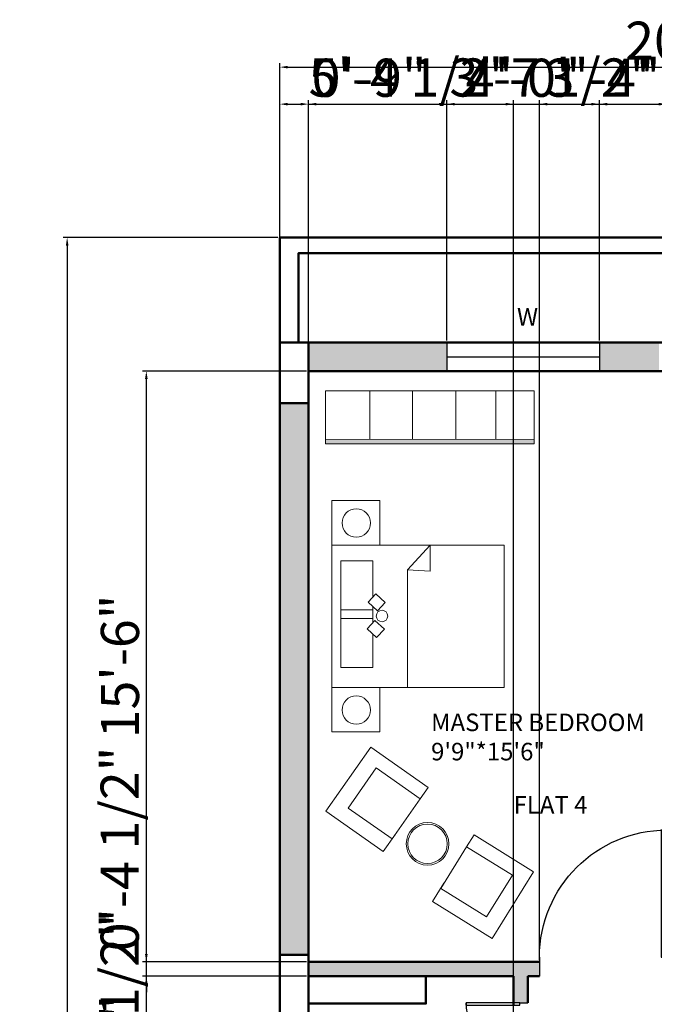
# Model space of a CAD drawing. Units: inches. Extents: x 2063 to 3370, y 2091 to 2971.
# Tile 13 of 14: x 2986 to 3185, y 2623 to 2933. Entities that reach past the tile are written whole.
import ezdxf

# ---------------------------------------------------------------- set-up
doc = ezdxf.new("R2010")
doc.units = ezdxf.units.IN
for name, color, linetype, lineweight in [('A-ANNO-DIMS', 2, 'Continuous', 18), ('A-ANNO-TEXT', 7, 'Continuous', 18), ('A-AREA-IDEN', 3, 'Continuous', 18), ('A-COLS', 7, 'Continuous', 50), ('A-DOOR', 4, 'Continuous', 25), ('A-FURN', 8, 'Continuous', 18), ('A-GLAZ', 131, 'Continuous', 25), ('A-WALL', 7, 'Continuous', 50), ('A-WALL-PATT', 8, 'Continuous', 13)]:
    doc.layers.add(name, color=color, linetype=linetype, lineweight=lineweight)
doc.styles.get("Standard").update_dxf_attribs({"font": 'arial.ttf'})
doc.dimstyles.new('ISO-25', dxfattribs={"dimtxt": 12, "dimasz": 2.5, "dimexe": 1.25, "dimexo": 0.625, "dimtad": 1, "dimdec": 0, "dimlunit": 4, "dimtxsty": 'Standard', "dimcen": 2.5, "dimadec": 0, "dimazin": 0, "dimtfac": 1, "dimtdec": 0, "dimtmove": 0, "dimatfit": 3, "dimfxl": 1, "dimarcsym": 0})

# ---------------------------------------------------------------- blocks, each defined once
blk = doc.blocks.new('*D9')
at = {"layer": 'A-ANNO-DIMS', "color": 0, "lineweight": -2, "transparency": 16777216}
for p, q in [((3067.42, 2865.05), (3067.42, 2919.33)), ((3069.92, 2918.08), (3304.92, 2918.08)), ((3307.42, 2865.05), (3307.42, 2919.33))]:
    blk.add_line(p, q, dxfattribs=at)
at = {"layer": 'A-ANNO-DIMS', "color": 0, "transparency": 16777216}
for points in [[(3069.92, 2918.5), (3069.92, 2917.67), (3067.42, 2918.08)], [(3304.92, 2918.5), (3304.92, 2917.67), (3307.42, 2918.08)]]:
    blk.add_solid(points, dxfattribs=at)
at = {"layer": 'Defpoints', "color": 0, "transparency": 16777216}
for p in [(3307.42, 2918.08), (3067.42, 2864.43), (3307.42, 2864.43)]:
    blk.add_point(p, dxfattribs=at)
at = {"layer": 'A-ANNO-DIMS', "color": 0, "transparency": 16777216, "insert": (3187.42, 2924.84), "char_height": 12, "attachment_point": 5}
blk.add_mtext("20'", dxfattribs=at)
blk = doc.blocks.new('*D10')
at = {"layer": 'A-ANNO-DIMS', "color": 0, "lineweight": -2, "transparency": 16777216}
for p, q in [((3066.79, 2864.43), (2999.25, 2864.43)), ((3000.5, 2861.93), (3000.5, 2146.93)), ((3066.79, 2144.43), (2999.25, 2144.43))]:
    blk.add_line(p, q, dxfattribs=at)
at = {"layer": 'A-ANNO-DIMS', "color": 0, "transparency": 16777216}
for points in [[(3000.09, 2861.93), (3000.92, 2861.93), (3000.5, 2864.43)], [(3000.09, 2146.93), (3000.92, 2146.93), (3000.5, 2144.43)]]:
    blk.add_solid(points, dxfattribs=at)
at = {"layer": 'Defpoints', "color": 0, "transparency": 16777216}
for p in [(3067.42, 2864.43), (3000.5, 2144.43), (3067.42, 2144.43)]:
    blk.add_point(p, dxfattribs=at)
at = {"layer": 'A-ANNO-DIMS', "color": 0, "transparency": 16777216, "insert": (2993.75, 2504.43), "char_height": 12, "attachment_point": 5, "rotation": 90}
blk.add_mtext("60'", dxfattribs=at)
blk = doc.blocks.new('*U2')
for p, q in [((0, 0), (0, -6)), ((40, 0), (40, -6))]:
    blk.add_line(p, q)
blk.add_lwpolyline([(0, 0), (0, 40), (1.75, 40), (1.75, 0)], close=True)
blk.add_arc((0, 0), 40, 0, 90)
blk = doc.blocks.new('BED-DOUBLE')
for p, q in [((23.79, 50.98), (30.96, 58.78)), ((30.96, 58.78), (30.96, 50.54)), ((23.79, 14), (23.79, 50.98)), ((30.96, 50.54), (23.79, 50.98))]:
    blk.add_line(p, q)
for points in [[(0, 58.78), (15.11, 58.78), (15.11, 72.78), (0, 72.78)], [(0, 58.78), (54.26, 58.78), (54.26, 14), (0, 14)], [(11.45, 40.86), (13.89, 43.46), (16.84, 40.71), (14.4, 38.1)], [(11.16, 32.43), (13.59, 35.03), (16.54, 32.28), (14.11, 29.67)], [(0, 0), (15.11, 0), (15.11, 14), (0, 14)]]:
    blk.add_lwpolyline(points, close=True)
for points in [[(12.88, 42.39), (12.88, 53.87), (2.9, 53.87), (2.9, 35.71), (12.88, 35.71), (12.88, 39.52)], [(12.88, 34.27), (12.88, 38.39), (2.9, 38.39), (2.9, 20.23), (12.88, 20.23), (12.88, 30.81)]]:
    blk.add_lwpolyline(points)
for centre, radius in [((7.71, 65.74), 4.47), ((15.81, 36.46), 1.81), ((7.71, 6.86), 4.47)]:
    blk.add_circle(centre, radius)
blk = doc.blocks.new('WARDROBE')
for p, q in [((13.88, 1.44), (13.88, 16.75)), ((27.33, 1.44), (27.33, 16.75)), ((40.97, 1.44), (40.97, 16.75)), ((53.56, 1.44), (53.56, 16.75)), ((0, 1.42), (65.55, 1.52))]:
    blk.add_line(p, q)
blk.add_lwpolyline([(0, 16.75), (65.55, 16.75), (65.55, 0), (0, 0)], close=True)
blk = doc.blocks.new('ARMCHAIR')
for p, q in [((10.7, 28.87), (13.03, 32.61)), ((13.03, 32.61), (31.78, 20.96)), ((31.78, 20.96), (18.75, 0)), ((0, 11.65), (3.54, 17.35)), ((18.75, 0), (0, 11.65))]:
    blk.add_line(p, q)
blk.add_lwpolyline([(2.55, 15.75), (16.92, 6.82), (25.07, 19.93), (10.7, 28.87)], close=True)
blk = doc.blocks.new('*D135')
at = {"layer": 'A-ANNO-DIMS', "color": 0, "lineweight": -2, "transparency": 16777216}
for p, q in [((3067.42, 2832.05), (3067.42, 2907.68)), ((3076.42, 2823.05), (3076.42, 2907.68)), ((3069.92, 2906.43), (3073.92, 2906.43)), ((3076.42, 2906.43), (3112.06, 2906.43))]:
    blk.add_line(p, q, dxfattribs=at)
at = {"layer": 'A-ANNO-DIMS', "color": 0, "transparency": 16777216}
for points in [[(3069.92, 2906.84), (3069.92, 2906.01), (3067.42, 2906.43)], [(3073.92, 2906.84), (3073.92, 2906.01), (3076.42, 2906.43)]]:
    blk.add_solid(points, dxfattribs=at)
at = {"layer": 'Defpoints', "color": 0, "transparency": 16777216}
for p in [(3076.42, 2906.43), (3067.42, 2831.43), (3076.42, 2822.43)]:
    blk.add_point(p, dxfattribs=at)
at = {"layer": 'A-ANNO-DIMS', "color": 0, "transparency": 16777216, "insert": (3095.49, 2913.18), "char_height": 12, "attachment_point": 5}
blk.add_mtext('0\'-9"', dxfattribs=at)
blk = doc.blocks.new('*D136')
at = {"layer": 'A-ANNO-DIMS', "color": 0, "lineweight": -2, "transparency": 16777216}
for p, q in [((3076.42, 2823.05), (3076.42, 2907.68)), ((3119.94, 2832.05), (3119.94, 2907.68)), ((3078.92, 2906.43), (3117.44, 2906.43)), ((3119.94, 2906.43), (3183.54, 2906.43))]:
    blk.add_line(p, q, dxfattribs=at)
at = {"layer": 'A-ANNO-DIMS', "color": 0, "transparency": 16777216}
for points in [[(3078.92, 2906.84), (3078.92, 2906.01), (3076.42, 2906.43)], [(3117.44, 2906.84), (3117.44, 2906.01), (3119.94, 2906.43)]]:
    blk.add_solid(points, dxfattribs=at)
at = {"layer": 'Defpoints', "color": 0, "transparency": 16777216}
for p in [(3119.94, 2906.43), (3119.94, 2831.43), (3076.42, 2822.43)]:
    blk.add_point(p, dxfattribs=at)
at = {"layer": 'A-ANNO-DIMS', "color": 0, "transparency": 16777216, "insert": (3152.99, 2913.26), "char_height": 12, "attachment_point": 5}
blk.add_mtext('3\'-7 1/2"', dxfattribs=at)
blk = doc.blocks.new('*D137')
at = {"layer": 'A-ANNO-DIMS', "color": 0, "lineweight": -2, "transparency": 16777216}
for p, q in [((3119.94, 2832.05), (3119.94, 2907.68)), ((3167.94, 2832.05), (3167.94, 2907.68)), ((3122.44, 2906.43), (3165.44, 2906.43))]:
    blk.add_line(p, q, dxfattribs=at)
at = {"layer": 'A-ANNO-DIMS', "color": 0, "transparency": 16777216}
for points in [[(3122.44, 2906.84), (3122.44, 2906.01), (3119.94, 2906.43)], [(3165.44, 2906.84), (3165.44, 2906.01), (3167.94, 2906.43)]]:
    blk.add_solid(points, dxfattribs=at)
at = {"layer": 'Defpoints', "color": 0, "transparency": 16777216}
for p in [(3167.94, 2906.43), (3119.94, 2831.43), (3167.94, 2831.43)]:
    blk.add_point(p, dxfattribs=at)
at = {"layer": 'A-ANNO-DIMS', "color": 0, "transparency": 16777216, "insert": (3143.94, 2913.18), "char_height": 12, "attachment_point": 5}
blk.add_mtext('4\'-0"', dxfattribs=at)
blk = doc.blocks.new('*D138')
at = {"layer": 'A-ANNO-DIMS', "color": 0, "lineweight": -2, "transparency": 16777216}
for p, q in [((3167.94, 2832.05), (3167.94, 2907.68)), ((3193.42, 2823.05), (3193.42, 2907.68)), ((3170.44, 2906.43), (3190.92, 2906.43)), ((3193.42, 2906.43), (3257.23, 2906.43))]:
    blk.add_line(p, q, dxfattribs=at)
at = {"layer": 'A-ANNO-DIMS', "color": 0, "transparency": 16777216}
for points in [[(3170.44, 2906.84), (3170.44, 2906.01), (3167.94, 2906.43)], [(3190.92, 2906.84), (3190.92, 2906.01), (3193.42, 2906.43)]]:
    blk.add_solid(points, dxfattribs=at)
at = {"layer": 'Defpoints', "color": 0, "transparency": 16777216}
for p in [(3193.42, 2906.43), (3167.94, 2831.43), (3193.42, 2822.43)]:
    blk.add_point(p, dxfattribs=at)
at = {"layer": 'A-ANNO-DIMS', "color": 0, "transparency": 16777216, "insert": (3226.57, 2913.26), "char_height": 12, "attachment_point": 5}
blk.add_mtext('2\'-1 1/2"', dxfattribs=at)
blk = doc.blocks.new('*D148')
at = {"layer": 'A-ANNO-DIMS', "color": 0, "lineweight": -2, "transparency": 16777216}
for p, q in [((3076.42, 2584.55), (3076.42, 2907.68)), ((3140.92, 2584.55), (3140.92, 2907.68)), ((3078.92, 2906.43), (3138.42, 2906.43))]:
    blk.add_line(p, q, dxfattribs=at)
at = {"layer": 'A-ANNO-DIMS', "color": 0, "transparency": 16777216}
for points in [[(3078.92, 2906.84), (3078.92, 2906.01), (3076.42, 2906.43)], [(3138.42, 2906.84), (3138.42, 2906.01), (3140.92, 2906.43)]]:
    blk.add_solid(points, dxfattribs=at)
at = {"layer": 'Defpoints', "color": 0, "transparency": 16777216}
for p in [(3140.92, 2906.43), (3076.42, 2583.93), (3140.92, 2583.93)]:
    blk.add_point(p, dxfattribs=at)
at = {"layer": 'A-ANNO-DIMS', "color": 0, "transparency": 16777216, "insert": (3108.67, 2913.26), "char_height": 12, "attachment_point": 5}
blk.add_mtext('5\'-4 1/2"', dxfattribs=at)
blk = doc.blocks.new('*D156')
at = {"layer": 'A-ANNO-DIMS', "color": 0, "lineweight": -2, "transparency": 16777216}
for p, q in [((3025.42, 2586.43), (3025.42, 2650.04)), ((3075.79, 2583.93), (3024.17, 2583.93)), ((3025.42, 2579.43), (3025.42, 2583.93)), ((3075.79, 2579.43), (3024.17, 2579.43)), ((3025.42, 2576.93), (3025.42, 2574.43))]:
    blk.add_line(p, q, dxfattribs=at)
at = {"layer": 'A-ANNO-DIMS', "color": 0, "transparency": 16777216}
for points in [[(3025, 2586.43), (3025.83, 2586.43), (3025.42, 2583.93)], [(3025, 2576.93), (3025.83, 2576.93), (3025.42, 2579.43)]]:
    blk.add_solid(points, dxfattribs=at)
at = {"layer": 'Defpoints', "color": 0, "transparency": 16777216}
for p in [(3025.42, 2583.93), (3076.42, 2583.93), (3076.42, 2579.43)]:
    blk.add_point(p, dxfattribs=at)
at = {"layer": 'A-ANNO-DIMS', "color": 0, "transparency": 16777216, "insert": (3018.59, 2619.48), "char_height": 12, "attachment_point": 5, "rotation": 90}
blk.add_mtext('0\'-4 1/2"', dxfattribs=at)
blk = doc.blocks.new('*D157')
at = {"layer": 'A-ANNO-DIMS', "color": 0, "lineweight": -2, "transparency": 16777216}
for p, q in [((3075.79, 2631.93), (3024.17, 2631.93)), ((3025.42, 2586.43), (3025.42, 2629.43)), ((3075.79, 2583.93), (3024.17, 2583.93))]:
    blk.add_line(p, q, dxfattribs=at)
at = {"layer": 'A-ANNO-DIMS', "color": 0, "transparency": 16777216}
for points in [[(3025, 2629.43), (3025.83, 2629.43), (3025.42, 2631.93)], [(3025, 2586.43), (3025.83, 2586.43), (3025.42, 2583.93)]]:
    blk.add_solid(points, dxfattribs=at)
at = {"layer": 'Defpoints', "color": 0, "transparency": 16777216}
for p in [(3025.42, 2631.93), (3076.42, 2631.93), (3076.42, 2583.93)]:
    blk.add_point(p, dxfattribs=at)
at = {"layer": 'A-ANNO-DIMS', "color": 0, "transparency": 16777216, "insert": (3018.66, 2607.93), "char_height": 12, "attachment_point": 5, "rotation": 90}
blk.add_mtext('4\'-0"', dxfattribs=at)
blk = doc.blocks.new('*D158')
at = {"layer": 'A-ANNO-DIMS', "color": 0, "lineweight": -2, "transparency": 16777216}
for p, q in [((3025.42, 2638.93), (3025.42, 2702.54)), ((3075.79, 2636.43), (3024.17, 2636.43)), ((3025.42, 2631.93), (3025.42, 2636.43)), ((3075.79, 2631.93), (3024.17, 2631.93)), ((3025.42, 2629.43), (3025.42, 2626.93))]:
    blk.add_line(p, q, dxfattribs=at)
at = {"layer": 'A-ANNO-DIMS', "color": 0, "transparency": 16777216}
for points in [[(3025, 2638.93), (3025.83, 2638.93), (3025.42, 2636.43)], [(3025, 2629.43), (3025.83, 2629.43), (3025.42, 2631.93)]]:
    blk.add_solid(points, dxfattribs=at)
at = {"layer": 'Defpoints', "color": 0, "transparency": 16777216}
for p in [(3025.42, 2636.43), (3076.42, 2636.43), (3076.42, 2631.93)]:
    blk.add_point(p, dxfattribs=at)
at = {"layer": 'A-ANNO-DIMS', "color": 0, "transparency": 16777216, "insert": (3018.59, 2671.98), "char_height": 12, "attachment_point": 5, "rotation": 90}
blk.add_mtext('0\'-4 1/2"', dxfattribs=at)
blk = doc.blocks.new('*D159')
at = {"layer": 'A-ANNO-DIMS', "color": 0, "lineweight": -2, "transparency": 16777216}
for p, q in [((3075.79, 2822.43), (3024.17, 2822.43)), ((3025.42, 2638.93), (3025.42, 2819.93)), ((3075.79, 2636.43), (3024.17, 2636.43))]:
    blk.add_line(p, q, dxfattribs=at)
at = {"layer": 'A-ANNO-DIMS', "color": 0, "transparency": 16777216}
for points in [[(3025, 2819.93), (3025.83, 2819.93), (3025.42, 2822.43)], [(3025, 2638.93), (3025.83, 2638.93), (3025.42, 2636.43)]]:
    blk.add_solid(points, dxfattribs=at)
at = {"layer": 'Defpoints', "color": 0, "transparency": 16777216}
for p in [(3025.42, 2822.43), (3076.42, 2822.43), (3076.42, 2636.43)]:
    blk.add_point(p, dxfattribs=at)
at = {"layer": 'A-ANNO-DIMS', "color": 0, "transparency": 16777216, "insert": (3018.66, 2729.43), "char_height": 12, "attachment_point": 5, "rotation": 90}
blk.add_mtext('15\'-6"', dxfattribs=at)
blk = doc.blocks.new('*D173')
at = {"layer": 'A-ANNO-DIMS', "color": 0, "lineweight": -2, "transparency": 16777216}
for p, q in [((3149.1, 2637.05), (3149.1, 2907.68)), ((3189.1, 2632.55), (3189.1, 2907.68)), ((3151.6, 2906.43), (3186.6, 2906.43))]:
    blk.add_line(p, q, dxfattribs=at)
at = {"layer": 'A-ANNO-DIMS', "color": 0, "transparency": 16777216}
for points in [[(3151.6, 2906.84), (3151.6, 2906.01), (3149.1, 2906.43)], [(3186.6, 2906.84), (3186.6, 2906.01), (3189.1, 2906.43)]]:
    blk.add_solid(points, dxfattribs=at)
at = {"layer": 'Defpoints', "color": 0, "transparency": 16777216}
for p in [(3189.1, 2906.43), (3149.1, 2636.43), (3189.1, 2631.93)]:
    blk.add_point(p, dxfattribs=at)
at = {"layer": 'A-ANNO-DIMS', "color": 0, "transparency": 16777216, "insert": (3169.1, 2913.18), "char_height": 12, "attachment_point": 5}
blk.add_mtext('3\'-4"', dxfattribs=at)

msp = doc.modelspace()

# ---------------------------------------------------------------- hatches: boundary and pattern name
at = {"layer": 'A-FURN'}
h = msp.add_hatch(color=256, dxfattribs=at)
h.dxf.hatch_style = 1
h.paths.add_polyline_path([(3147.38, 2800.98), (3081.83, 2800.89), (3081.83, 2799.47), (3147.38, 2799.47)])
at = {"layer": 'A-WALL-PATT'}
h = msp.add_hatch(color=256, dxfattribs=at)
h.dxf.hatch_style = 1
h.paths.add_polyline_path([(3181.8, 2234.43), (3076.42, 2234.43), (3076.42, 2232.93), (3076.42, 2225.43), (3181.8, 2225.43)])
h.paths.add_polyline_path([(3212.92, 2192.43), (3200.92, 2192.43), (3104.92, 2192.43), (3104.92, 2189.43), (3104.92, 2187.43), (3200.92, 2187.43), (3212.92, 2187.42)], flags=17)
h.paths.add_polyline_path([(3219.45, 2153.43), (3076.42, 2153.43), (3076.42, 2222.57), (3067.42, 2222.57), (3067.42, 2144.43), (3219.45, 2144.43)])
h.paths.add_polyline_path([(3076.42, 2343.93), (3076.42, 2351.28), (3067.42, 2351.28), (3067.42, 2241.68), (3076.42, 2241.68), (3076.42, 2258.43)])
h.paths.add_polyline_path([(3175.73, 2554.94), (3230.21, 2554.94), (3230.21, 2575.54), (3175.73, 2575.54)], flags=9)
h.paths.add_polyline_path([(3085.27, 2530.92), (3121.9, 2530.92), (3121.9, 2551.53), (3085.27, 2551.53)], flags=9)
h.paths.add_polyline_path([(3089.9, 2596.23), (3114.49, 2596.23), (3114.49, 2616.83), (3089.9, 2616.83)], flags=9)
h.paths.add_polyline_path([(3260.79, 2797.55), (3297.86, 2797.55), (3297.86, 2808.94), (3260.79, 2808.94)], flags=9)
h.paths.add_polyline_path([(3113.05, 2696.74), (3189.97, 2696.74), (3189.97, 2717.35), (3113.05, 2717.35)], flags=9)
h.paths.add_polyline_path([(3226.64, 2835.24), (3234.55, 2835.24), (3234.55, 2846.62), (3226.64, 2846.62)], flags=9)
h.paths.add_polyline_path([(3140.56, 2833.68), (3150.6, 2833.68), (3150.6, 2845.06), (3140.56, 2845.06)], flags=9)
h.paths.add_polyline_path([(3193.53, 2795.64), (3230.6, 2795.64), (3230.6, 2807.02), (3193.53, 2807.02)], flags=9)
h.paths.add_polyline_path([(3225.05, 2726.09), (3287.83, 2726.09), (3287.83, 2746.7), (3225.05, 2746.7)], flags=9)
h = msp.add_hatch(color=256, dxfattribs=at)
h.dxf.hatch_style = 1
h.paths.add_polyline_path([(3294.05, 2153.43), (3219.45, 2153.43), (3219.45, 2144.43), (3294.05, 2144.43)])
h.paths.add_polyline_path([(3307.42, 2220.3), (3298.42, 2220.3), (3298.42, 2153.43), (3294.05, 2153.43), (3294.05, 2144.43), (3307.42, 2144.43)])
h.paths.add_polyline_path([(3076.42, 2468.43), (3076.42, 2477.43), (3076.42, 2514.15), (3067.42, 2514.15), (3067.42, 2370.39), (3076.42, 2370.39)])
h.paths.add_polyline_path([(3307.42, 2525.28), (3298.42, 2525.28), (3298.42, 2523.93), (3298.42, 2466.93), (3298.42, 2383.04), (3307.42, 2383.04)])
h.paths.add_polyline_path([(3307.42, 2363.93), (3298.42, 2363.93), (3298.42, 2239.41), (3307.42, 2239.41)])
h.paths.add_polyline_path([(3235.32, 2180.53), (3274.95, 2180.53), (3274.95, 2201.14), (3235.32, 2201.14)], flags=9)
h.paths.add_polyline_path([(3127.74, 2323.36), (3191.84, 2323.36), (3191.84, 2343.96), (3127.74, 2343.96)], flags=9)
h.paths.add_polyline_path([(3175.73, 2554.94), (3230.21, 2554.94), (3230.21, 2575.54), (3175.73, 2575.54)], flags=9)
h.paths.add_polyline_path([(3085.27, 2530.92), (3121.9, 2530.92), (3121.9, 2551.53), (3085.27, 2551.53)], flags=9)
h.paths.add_polyline_path([(3089.9, 2596.23), (3114.49, 2596.23), (3114.49, 2616.83), (3089.9, 2616.83)], flags=9)
h.paths.add_polyline_path([(3260.79, 2797.55), (3297.86, 2797.55), (3297.86, 2808.94), (3260.79, 2808.94)], flags=9)
h.paths.add_polyline_path([(3113.05, 2696.74), (3189.97, 2696.74), (3189.97, 2717.35), (3113.05, 2717.35)], flags=9)
h.paths.add_polyline_path([(3226.64, 2835.24), (3234.55, 2835.24), (3234.55, 2846.62), (3226.64, 2846.62)], flags=9)
h.paths.add_polyline_path([(3140.56, 2833.68), (3150.6, 2833.68), (3150.6, 2845.06), (3140.56, 2845.06)], flags=9)
h.paths.add_polyline_path([(3193.53, 2795.64), (3230.6, 2795.64), (3230.6, 2807.02), (3193.53, 2807.02)], flags=9)
h.paths.add_polyline_path([(3225.05, 2726.09), (3287.83, 2726.09), (3287.83, 2746.7), (3225.05, 2746.7)], flags=9)
h = msp.add_hatch(color=256, dxfattribs=at)
h.dxf.hatch_style = 1
h.paths.add_polyline_path([(3076.42, 2619.52), (3067.42, 2619.52), (3067.42, 2548.5), (3076.42, 2548.5), (3076.42, 2579.43)])
h.paths.add_polyline_path([(3236.69, 2636.43), (3197.92, 2636.43), (3197.92, 2631.93), (3236.69, 2631.93)])
h.paths.add_polyline_path([(3145.42, 2631.93), (3149.1, 2631.93), (3149.1, 2636.43), (3147.77, 2636.43), (3076.42, 2636.43), (3076.42, 2631.93), (3113.39, 2631.93), (3136.42, 2631.93), (3140.92, 2631.93), (3140.92, 2623.58), (3142.89, 2623.58), (3145.42, 2623.58)])
h.paths.add_polyline_path([(3298.42, 2636.43), (3276.69, 2636.43), (3276.69, 2631.93), (3298.42, 2631.93)])
h.paths.add_polyline_path([(3307.42, 2679.03), (3298.42, 2679.03), (3298.42, 2645.28), (3307.42, 2645.28)])
h.paths.add_polyline_path([(3307.42, 2626.16), (3298.42, 2626.16), (3298.42, 2585.28), (3307.42, 2585.28)])
h.paths.add_polyline_path([(3260.79, 2797.55), (3297.86, 2797.55), (3297.86, 2808.94), (3260.79, 2808.94)], flags=9)
h.paths.add_polyline_path([(3113.05, 2696.74), (3189.97, 2696.74), (3189.97, 2717.35), (3113.05, 2717.35)], flags=9)
h.paths.add_polyline_path([(3226.64, 2835.24), (3234.55, 2835.24), (3234.55, 2846.62), (3226.64, 2846.62)], flags=9)
h.paths.add_polyline_path([(3140.56, 2833.68), (3150.6, 2833.68), (3150.6, 2845.06), (3140.56, 2845.06)], flags=9)
h.paths.add_polyline_path([(3193.53, 2795.64), (3230.6, 2795.64), (3230.6, 2807.02), (3193.53, 2807.02)], flags=9)
h.paths.add_polyline_path([(3225.05, 2726.09), (3287.83, 2726.09), (3287.83, 2746.7), (3225.05, 2746.7)], flags=9)
h = msp.add_hatch(color=256, dxfattribs=at)
h.dxf.hatch_style = 1
h.paths.add_polyline_path([(3119.94, 2831.43), (3076.42, 2831.43), (3076.42, 2822.43), (3119.94, 2822.43)])
h.paths.add_polyline_path([(3186.73, 2831.43), (3167.94, 2831.43), (3167.94, 2822.43), (3186.73, 2822.43)])
h.paths.add_polyline_path([(3219.33, 2831.43), (3205.84, 2831.43), (3205.84, 2822.43), (3219.33, 2822.43)])
h.paths.add_polyline_path([(3298.42, 2831.43), (3243.76, 2831.43), (3243.76, 2822.43), (3298.42, 2822.43)])
h.paths.add_polyline_path([(3235.32, 2180.53), (3274.95, 2180.53), (3274.95, 2201.14), (3235.32, 2201.14)], flags=9)
h.paths.add_polyline_path([(3127.74, 2323.36), (3191.84, 2323.36), (3191.84, 2343.96), (3127.74, 2343.96)], flags=9)
h.paths.add_polyline_path([(3175.73, 2554.94), (3230.21, 2554.94), (3230.21, 2575.54), (3175.73, 2575.54)], flags=9)
h.paths.add_polyline_path([(3085.27, 2530.92), (3121.9, 2530.92), (3121.9, 2551.53), (3085.27, 2551.53)], flags=9)
h.paths.add_polyline_path([(3089.9, 2596.23), (3114.49, 2596.23), (3114.49, 2616.83), (3089.9, 2616.83)], flags=9)
h.paths.add_polyline_path([(3113.05, 2696.74), (3189.97, 2696.74), (3189.97, 2717.35), (3113.05, 2717.35)], flags=9)
h.paths.add_polyline_path([(3193.53, 2795.64), (3230.6, 2795.64), (3230.6, 2807.02), (3193.53, 2807.02)], flags=9)
h.paths.add_polyline_path([(3225.05, 2726.09), (3287.83, 2726.09), (3287.83, 2746.7), (3225.05, 2746.7)], flags=9)
h = msp.add_hatch(color=256, dxfattribs=at)
h.dxf.hatch_style = 1
h.paths.add_polyline_path([(3076.42, 2812.31), (3067.42, 2812.31), (3067.42, 2638.63), (3076.42, 2638.63)])
h = msp.add_hatch(color=256, dxfattribs=at)
h.dxf.hatch_style = 1
h.paths.add_polyline_path([(3254.4, 2477.43), (3145.42, 2477.43), (3145.42, 2579.43), (3145.42, 2589.96), (3142.89, 2589.96), (3140.92, 2589.96), (3140.92, 2583.93), (3131.92, 2583.93), (3076.42, 2583.93), (3076.42, 2579.43), (3136.42, 2579.43), (3140.92, 2579.43), (3140.92, 2477.43), (3076.42, 2477.43), (3076.42, 2468.43), (3193.42, 2468.43), (3254.4, 2468.43), (3254.4, 2471.41)])
h.paths.add_polyline_path([(3235.32, 2180.53), (3274.95, 2180.53), (3274.95, 2201.14), (3235.32, 2201.14)], flags=9)
h.paths.add_polyline_path([(3127.74, 2323.36), (3191.84, 2323.36), (3191.84, 2343.96), (3127.74, 2343.96)], flags=9)
h.paths.add_polyline_path([(3175.73, 2554.94), (3230.21, 2554.94), (3230.21, 2575.54), (3175.73, 2575.54)], flags=25)
h.paths.add_polyline_path([(3089.9, 2596.23), (3114.49, 2596.23), (3114.49, 2616.83), (3089.9, 2616.83)], flags=9)
h.paths.add_polyline_path([(3260.79, 2797.55), (3297.86, 2797.55), (3297.86, 2808.94), (3260.79, 2808.94)], flags=9)
h.paths.add_polyline_path([(3113.05, 2696.74), (3189.97, 2696.74), (3189.97, 2717.35), (3113.05, 2717.35)], flags=9)
h.paths.add_polyline_path([(3193.53, 2795.64), (3230.6, 2795.64), (3230.6, 2807.02), (3193.53, 2807.02)], flags=9)
h.paths.add_polyline_path([(3225.05, 2726.09), (3287.83, 2726.09), (3287.83, 2746.7), (3225.05, 2746.7)], flags=9)

# ---------------------------------------------------------------- linework, layer by layer
at = {"layer": 'A-COLS'}
for points in [[(3067.42, 2831.43), (3076.42, 2831.43), (3076.42, 2812.31), (3067.42, 2812.31)], [(3067.42, 2638.63), (3076.42, 2638.63), (3076.42, 2619.52), (3067.42, 2619.52)]]:
    msp.add_lwpolyline(points, close=True, dxfattribs=at)
at = {"layer": 'A-FURN'}
for radius in [6.72, 6.2]:
    msp.add_circle((3113.9, 2673.62), radius, dxfattribs=at)
at = {"layer": 'A-GLAZ'}
for p, q in [((3119.94, 2831.43), (3119.94, 2822.43)), ((3167.94, 2831.43), (3167.94, 2822.43)), ((3119.94, 2826.93), (3167.94, 2826.93))]:
    msp.add_line(p, q, dxfattribs=at)
at = {"layer": 'A-WALL'}
for p, q in [((3076.42, 2822.43), (3193.42, 2822.43)), ((3076.42, 2822.43), (3193.42, 2822.43)), ((3076.42, 2636.43), (3147.77, 2636.43)), ((3147.77, 2636.43), (3149.1, 2636.43)), ((3076.42, 2631.93), (3136.42, 2631.93)), ((3076.42, 2631.93), (3136.42, 2631.93)), ((3136.42, 2631.93), (3140.92, 2631.93)), ((3140.92, 2622.85), (3140.92, 2631.93)), ((3145.42, 2631.93), (3147.77, 2631.93)), ((3145.42, 2623.58), (3145.42, 2631.93)), ((3145.42, 2631.93), (3149.1, 2631.93))]:
    msp.add_line(p, q, dxfattribs=at)
for points in [[(3067.42, 2144.43), (3307.42, 2144.43), (3307.42, 2864.43), (3067.42, 2864.43)], [(3301.03, 2831.43), (3301.03, 2859.54), (3073.29, 2859.54), (3073.29, 2831.43)], [(3076.42, 2631.93), (3113.39, 2631.93), (3113.39, 2623.33), (3076.42, 2623.33)]]:
    msp.add_lwpolyline(points, close=True, dxfattribs=at)
for points in [[(3076.42, 2822.43), (3076.42, 2576.43)], [(3076.42, 2631.93), (3076.42, 2583.93)]]:
    msp.add_lwpolyline(points, dxfattribs=at)

# ---------------------------------------------------------------- block references
at = {"layer": 'A-DOOR', "xscale": -1}
msp.add_blockref('*U2', (3189.1, 2637.93), dxfattribs=at)
at = {"layer": 'A-DOOR', "xscale": -0.4203428619043682, "yscale": 0.4203428619043682, "zscale": 0.4203428619043682, "rotation": 90}
msp.add_blockref('*U2', (3142.89, 2623.58), dxfattribs=at)
at = {"layer": 'A-FURN'}
for name, p in [('WARDROBE', (3081.83, 2799.47)), ('BED-DOUBLE', (3083.75, 2708.85)), ('ARMCHAIR', (3115.49, 2643.83))]:
    msp.add_blockref(name, p, dxfattribs=at)
at = {"layer": 'A-FURN', "extrusion": (0, 0, -1), "zscale": -1, "rotation": 66.95512356980076}
msp.add_blockref('ARMCHAIR', (-3089.22, 2666.62), dxfattribs=at)

# ---------------------------------------------------------------- texts
at = {"layer": 'A-ANNO-TEXT', "attachment_point": 1}
for s, heights, insert, char_height in [('W', [0], (3142.03, 2842.22), 5.52), ('FLAT 4', [14.84], (3140.97, 2688.65), 5.523)]:
    msp.add_mtext_dynamic_manual_height_columns(s, width=106.0361, gutter_width=27.61, heights=heights, dxfattribs=dict(at, insert=insert, char_height=char_height))
at = {"layer": 'A-AREA-IDEN', "insert": (3115, 2714.6), "char_height": 5.5229, "attachment_point": 1}
msp.add_mtext_dynamic_manual_height_columns('MASTER BEDROOM\\P9\'9"*15\'6"', width=106.0361, gutter_width=27.61, heights=[0], dxfattribs=at)

# ---------------------------------------------------------------- dimensions: what is measured, and where the dimension line sits
at = {"layer": 'A-ANNO-DIMS'}
for base, p1, p2, override, picture, middle in [((3307.42, 2918.08), (3067.42, 2864.43), (3307.42, 2864.43), {"dimclrd": 0, "dimclre": 0, "dimclrt": 0}, '*D9', (3187.42, 2924.84)), ((3119.94, 2906.43), (3076.42, 2822.43), (3119.94, 2831.43), {"dimdec": 1, "dimlfac": 1, "dimrnd": 0, "dimzin": 1, "dimdsep": 46, "dimlunit": 4, "dimfrac": 2}, '*D136', (3152.99, 2913.26)), ((3140.92, 2906.43), (3076.42, 2583.93), (3140.92, 2583.93), {"dimdec": 1, "dimlfac": 1, "dimrnd": 0, "dimzin": 1, "dimdsep": 46, "dimlunit": 4, "dimfrac": 2}, '*D148', (3108.67, 2913.26)), ((3193.42, 2906.43), (3167.94, 2831.43), (3193.42, 2822.43), {"dimdec": 1, "dimlfac": 1, "dimrnd": 0, "dimzin": 1, "dimdsep": 46, "dimlunit": 4, "dimfrac": 2}, '*D138', (3226.57, 2913.26)), ((3076.42, 2906.43), (3067.42, 2831.43), (3076.42, 2822.43), {"dimdec": 1, "dimlfac": 1, "dimrnd": 0, "dimzin": 1, "dimdsep": 46, "dimlunit": 4, "dimfrac": 2}, '*D135', (3095.49, 2913.18)), ((3167.94, 2906.43), (3119.94, 2831.43), (3167.94, 2831.43), {"dimdec": 1, "dimlfac": 1, "dimrnd": 0, "dimzin": 1, "dimdsep": 46, "dimlunit": 4, "dimfrac": 2}, '*D137', (3143.94, 2913.18)), ((3189.1, 2906.43), (3149.1, 2636.43), (3189.1, 2631.93), {"dimdec": 1, "dimlfac": 1, "dimrnd": 0, "dimzin": 1, "dimdsep": 46, "dimlunit": 4, "dimfrac": 2}, '*D173', (3169.1, 2913.18))]:
    dim = msp.add_linear_dim(base=base, p1=p1, p2=p2, dimstyle='ISO-25', override=override, dxfattribs=at)
    dim.commit()
    dim.dimension.update_dxf_attribs({"geometry": picture, "text_midpoint": middle})
for base, p1, p2, override, picture, middle in [((3000.5, 2144.43), (3067.42, 2864.43), (3067.42, 2144.43), {"dimclrd": 0, "dimclre": 0, "dimclrt": 0}, '*D10', (2993.75, 2504.43)), ((3025.42, 2822.43), (3076.42, 2636.43), (3076.42, 2822.43), {"dimdec": 1, "dimlfac": 1, "dimrnd": 0, "dimzin": 1, "dimdsep": 46, "dimlunit": 4, "dimfrac": 2}, '*D159', (3018.66, 2729.43)), ((3025.42, 2636.43), (3076.42, 2631.93), (3076.42, 2636.43), {"dimdec": 1, "dimlfac": 1, "dimrnd": 0, "dimzin": 1, "dimdsep": 46, "dimlunit": 4, "dimfrac": 2}, '*D158', (3018.59, 2671.98)), ((3025.42, 2583.93), (3076.42, 2579.43), (3076.42, 2583.93), {"dimdec": 1, "dimlfac": 1, "dimrnd": 0, "dimzin": 1, "dimdsep": 46, "dimlunit": 4, "dimfrac": 2}, '*D156', (3018.59, 2619.48)), ((3025.42, 2631.93), (3076.42, 2583.93), (3076.42, 2631.93), {"dimdec": 1, "dimlfac": 1, "dimrnd": 0, "dimzin": 1, "dimdsep": 46, "dimlunit": 4, "dimfrac": 2}, '*D157', (3018.66, 2607.93))]:
    dim = msp.add_linear_dim(base=base, p1=p1, p2=p2, angle=90, dimstyle='ISO-25', override=override, dxfattribs=at)
    dim.commit()
    dim.dimension.update_dxf_attribs({"geometry": picture, "text_midpoint": middle})

doc.saveas('drawing.dxf')
